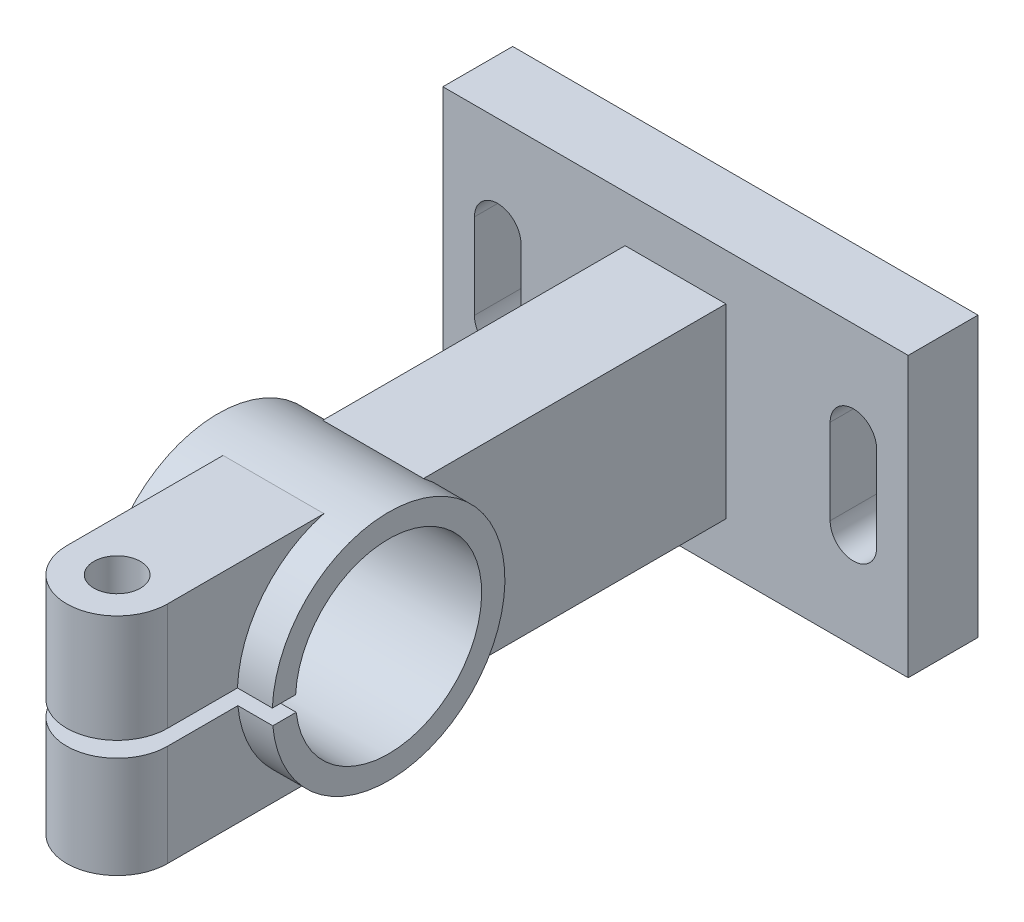
ISO-10303-21;
HEADER;
FILE_DESCRIPTION(('STEP AP214'),'2;1');
FILE_NAME('part.step','',(''),(''),'','','');
FILE_SCHEMA(('AUTOMOTIVE_DESIGN { 1 0 10303 214 1 1 1 1 }'));
ENDSEC;
DATA;
#1=APPLICATION_CONTEXT('core data for automotive mechanical design processes');
#2=APPLICATION_PROTOCOL_DEFINITION('international standard','automotive_design',2000,#1);
#3=PRODUCT_CONTEXT('',#1,'mechanical');
#4=PRODUCT('Part','Part','',(#3));
#5=PRODUCT_RELATED_PRODUCT_CATEGORY('part','',(#4));
#6=PRODUCT_DEFINITION_FORMATION('','',#4);
#7=PRODUCT_DEFINITION_CONTEXT('part definition',#1,'design');
#8=PRODUCT_DEFINITION('design','',#6,#7);
#9=PRODUCT_DEFINITION_SHAPE('','',#8);
#10=(LENGTH_UNIT() NAMED_UNIT(*) SI_UNIT(.MILLI.,.METRE.));
#11=(NAMED_UNIT(*) PLANE_ANGLE_UNIT() SI_UNIT($,.RADIAN.));
#12=(NAMED_UNIT(*) SI_UNIT($,.STERADIAN.) SOLID_ANGLE_UNIT());
#13=UNCERTAINTY_MEASURE_WITH_UNIT(LENGTH_MEASURE(1.E-05),#10,'distance_accuracy_value','');
#14=(GEOMETRIC_REPRESENTATION_CONTEXT(3) GLOBAL_UNCERTAINTY_ASSIGNED_CONTEXT((#13)) GLOBAL_UNIT_ASSIGNED_CONTEXT((#10,
#11,#12)) REPRESENTATION_CONTEXT('',''));
#15=CARTESIAN_POINT('',(0.,0.,0.));
#16=DIRECTION('',(0.,0.,1.));
#17=DIRECTION('',(1.,0.,0.));
#18=AXIS2_PLACEMENT_3D('',#15,#16,#17);
#19=CARTESIAN_POINT('',(0.,0.,9.));
#20=DIRECTION('',(0.,0.,-1.));
#21=DIRECTION('',(-1.,0.,0.));
#22=AXIS2_PLACEMENT_3D('',#19,#20,#21);
#23=PLANE('',#22);
#24=DIRECTION('',(0.,-1.,0.));
#25=VECTOR('',#24,1.);
#26=CARTESIAN_POINT('',(8.13242818806854,47.,9.));
#27=LINE('',#26,#25);
#28=CARTESIAN_POINT('',(8.13242818806854,47.,9.));
#29=VERTEX_POINT('',#28);
#30=CARTESIAN_POINT('',(8.13242818806854,25.,9.));
#31=VERTEX_POINT('',#30);
#32=EDGE_CURVE('E246',#29,#31,#27,.T.);
#33=ORIENTED_EDGE('',*,*,#32,.F.);
#34=CARTESIAN_POINT('',(14.1324281880685,47.,9.));
#35=DIRECTION('',(0.,0.,1.));
#36=DIRECTION('',(1.,0.,0.));
#37=AXIS2_PLACEMENT_3D('',#34,#35,#36);
#38=CIRCLE('',#37,6.);
#39=CARTESIAN_POINT('',(20.1324281880686,47.,9.));
#40=VERTEX_POINT('',#39);
#41=EDGE_CURVE('E58',#40,#29,#38,.T.);
#42=ORIENTED_EDGE('',*,*,#41,.F.);
#43=DIRECTION('',(0.,-1.,0.));
#44=VECTOR('',#43,1.);
#45=CARTESIAN_POINT('',(20.1324281880686,47.,9.));
#46=LINE('',#45,#44);
#47=CARTESIAN_POINT('',(20.1324281880686,25.,9.));
#48=VERTEX_POINT('',#47);
#49=EDGE_CURVE('E255',#40,#48,#46,.T.);
#50=ORIENTED_EDGE('',*,*,#49,.T.);
#51=CARTESIAN_POINT('',(14.1324281880685,25.,9.));
#52=DIRECTION('',(0.,0.,1.));
#53=DIRECTION('',(1.,0.,0.));
#54=AXIS2_PLACEMENT_3D('',#51,#52,#53);
#55=CIRCLE('',#54,6.);
#56=EDGE_CURVE('E236',#31,#48,#55,.T.);
#57=ORIENTED_EDGE('',*,*,#56,.F.);
#58=EDGE_LOOP('',(#33,#42,#50,#57));
#59=FACE_BOUND('',#58,.T.);
#60=DIRECTION('',(0.,-1.,0.));
#61=VECTOR('',#60,1.);
#62=CARTESIAN_POINT('',(47.,60.,9.));
#63=LINE('',#62,#61);
#64=CARTESIAN_POINT('',(47.,60.,9.));
#65=VERTEX_POINT('',#64);
#66=CARTESIAN_POINT('',(47.,12.,9.));
#67=VERTEX_POINT('',#66);
#68=EDGE_CURVE('E381',#65,#67,#63,.T.);
#69=ORIENTED_EDGE('',*,*,#68,.F.);
#70=DIRECTION('',(1.,0.,0.));
#71=VECTOR('',#70,1.);
#72=CARTESIAN_POINT('',(47.,60.,9.));
#73=LINE('',#72,#71);
#74=CARTESIAN_POINT('',(73.,60.,9.));
#75=VERTEX_POINT('',#74);
#76=EDGE_CURVE('E373',#65,#75,#73,.T.);
#77=ORIENTED_EDGE('',*,*,#76,.T.);
#78=DIRECTION('',(0.,-1.,0.));
#79=VECTOR('',#78,1.);
#80=CARTESIAN_POINT('',(73.,60.,9.));
#81=LINE('',#80,#79);
#82=CARTESIAN_POINT('',(73.,12.,9.));
#83=VERTEX_POINT('',#82);
#84=EDGE_CURVE('E374',#75,#83,#81,.T.);
#85=ORIENTED_EDGE('',*,*,#84,.T.);
#86=DIRECTION('',(1.,0.,0.));
#87=VECTOR('',#86,1.);
#88=CARTESIAN_POINT('',(47.,12.,9.));
#89=LINE('',#88,#87);
#90=EDGE_CURVE('E378',#67,#83,#89,.T.);
#91=ORIENTED_EDGE('',*,*,#90,.F.);
#92=EDGE_LOOP('',(#69,#77,#85,#91));
#93=FACE_BOUND('',#92,.T.);
#94=DIRECTION('',(0.,1.,0.));
#95=VECTOR('',#94,1.);
#96=CARTESIAN_POINT('',(0.,0.,9.));
#97=LINE('',#96,#95);
#98=CARTESIAN_POINT('',(0.,0.,9.));
#99=VERTEX_POINT('',#98);
#100=CARTESIAN_POINT('',(0.,72.,9.));
#101=VERTEX_POINT('',#100);
#102=EDGE_CURVE('E403',#99,#101,#97,.T.);
#103=ORIENTED_EDGE('',*,*,#102,.F.);
#104=DIRECTION('',(1.,0.,0.));
#105=VECTOR('',#104,1.);
#106=CARTESIAN_POINT('',(0.,0.,9.));
#107=LINE('',#106,#105);
#108=CARTESIAN_POINT('',(120.,0.,9.));
#109=VERTEX_POINT('',#108);
#110=EDGE_CURVE('E414',#99,#109,#107,.T.);
#111=ORIENTED_EDGE('',*,*,#110,.T.);
#112=DIRECTION('',(0.,1.,0.));
#113=VECTOR('',#112,1.);
#114=CARTESIAN_POINT('',(120.,0.,9.));
#115=LINE('',#114,#113);
#116=CARTESIAN_POINT('',(120.,72.,9.));
#117=VERTEX_POINT('',#116);
#118=EDGE_CURVE('E415',#109,#117,#115,.T.);
#119=ORIENTED_EDGE('',*,*,#118,.T.);
#120=DIRECTION('',(1.,0.,0.));
#121=VECTOR('',#120,1.);
#122=CARTESIAN_POINT('',(0.,72.,9.));
#123=LINE('',#122,#121);
#124=EDGE_CURVE('E409',#101,#117,#123,.T.);
#125=ORIENTED_EDGE('',*,*,#124,.F.);
#126=EDGE_LOOP('',(#103,#111,#119,#125));
#127=FACE_BOUND('',#126,.T.);
#128=CARTESIAN_POINT('',(105.867571811931,47.,9.));
#129=DIRECTION('',(0.,0.,-1.));
#130=DIRECTION('',(-1.,0.,0.));
#131=AXIS2_PLACEMENT_3D('',#128,#129,#130);
#132=CIRCLE('',#131,6.00000000000001);
#133=CARTESIAN_POINT('',(99.8675718119314,47.,9.));
#134=VERTEX_POINT('',#133);
#135=CARTESIAN_POINT('',(111.867571811931,47.,9.));
#136=VERTEX_POINT('',#135);
#137=EDGE_CURVE('E68',#134,#136,#132,.T.);
#138=ORIENTED_EDGE('',*,*,#137,.T.);
#139=DIRECTION('',(0.,-1.,0.));
#140=VECTOR('',#139,1.);
#141=CARTESIAN_POINT('',(111.867571811931,47.,9.));
#142=LINE('',#141,#140);
#143=CARTESIAN_POINT('',(111.867571811931,25.,9.));
#144=VERTEX_POINT('',#143);
#145=EDGE_CURVE('E277',#136,#144,#142,.T.);
#146=ORIENTED_EDGE('',*,*,#145,.T.);
#147=CARTESIAN_POINT('',(105.867571811931,25.,9.));
#148=DIRECTION('',(0.,0.,-1.));
#149=DIRECTION('',(-1.,0.,0.));
#150=AXIS2_PLACEMENT_3D('',#147,#148,#149);
#151=CIRCLE('',#150,6.00000000000001);
#152=CARTESIAN_POINT('',(99.8675718119314,25.,9.));
#153=VERTEX_POINT('',#152);
#154=EDGE_CURVE('E271',#144,#153,#151,.T.);
#155=ORIENTED_EDGE('',*,*,#154,.T.);
#156=DIRECTION('',(0.,-1.,0.));
#157=VECTOR('',#156,1.);
#158=CARTESIAN_POINT('',(99.8675718119314,47.,9.));
#159=LINE('',#158,#157);
#160=EDGE_CURVE('E268',#134,#153,#159,.T.);
#161=ORIENTED_EDGE('',*,*,#160,.F.);
#162=EDGE_LOOP('',(#138,#146,#155,#161));
#163=FACE_BOUND('',#162,.T.);
#164=ADVANCED_FACE('F44',(#59,#93,#127,#163),#23,.F.);
#165=CARTESIAN_POINT('',(0.,0.,-9.));
#166=DIRECTION('',(0.,0.,-1.));
#167=DIRECTION('',(-1.,0.,0.));
#168=AXIS2_PLACEMENT_3D('',#165,#166,#167);
#169=PLANE('',#168);
#170=CARTESIAN_POINT('',(14.1324281880685,47.,-9.));
#171=DIRECTION('',(0.,0.,-1.));
#172=DIRECTION('',(-1.,0.,0.));
#173=AXIS2_PLACEMENT_3D('',#170,#171,#172);
#174=CIRCLE('',#173,6.);
#175=CARTESIAN_POINT('',(8.13242818806854,47.,-9.));
#176=VERTEX_POINT('',#175);
#177=CARTESIAN_POINT('',(20.1324281880686,47.,-9.));
#178=VERTEX_POINT('',#177);
#179=EDGE_CURVE('E12',#176,#178,#174,.T.);
#180=ORIENTED_EDGE('',*,*,#179,.F.);
#181=DIRECTION('',(0.,1.,0.));
#182=VECTOR('',#181,1.);
#183=CARTESIAN_POINT('',(8.13242818806854,0.,-9.));
#184=LINE('',#183,#182);
#185=CARTESIAN_POINT('',(8.13242818806854,25.,-9.));
#186=VERTEX_POINT('',#185);
#187=EDGE_CURVE('E452',#186,#176,#184,.T.);
#188=ORIENTED_EDGE('',*,*,#187,.F.);
#189=CARTESIAN_POINT('',(14.1324281880685,25.,-9.));
#190=DIRECTION('',(0.,0.,-1.));
#191=DIRECTION('',(-1.,0.,0.));
#192=AXIS2_PLACEMENT_3D('',#189,#190,#191);
#193=CIRCLE('',#192,6.);
#194=CARTESIAN_POINT('',(20.1324281880686,25.,-9.));
#195=VERTEX_POINT('',#194);
#196=EDGE_CURVE('E237',#195,#186,#193,.T.);
#197=ORIENTED_EDGE('',*,*,#196,.F.);
#198=DIRECTION('',(0.,1.,0.));
#199=VECTOR('',#198,1.);
#200=CARTESIAN_POINT('',(20.1324281880686,0.,-9.));
#201=LINE('',#200,#199);
#202=EDGE_CURVE('E52',#195,#178,#201,.T.);
#203=ORIENTED_EDGE('',*,*,#202,.T.);
#204=EDGE_LOOP('',(#180,#188,#197,#203));
#205=FACE_BOUND('',#204,.T.);
#206=DIRECTION('',(0.,1.,0.));
#207=VECTOR('',#206,1.);
#208=CARTESIAN_POINT('',(0.,0.,-9.));
#209=LINE('',#208,#207);
#210=CARTESIAN_POINT('',(0.,0.,-9.));
#211=VERTEX_POINT('',#210);
#212=CARTESIAN_POINT('',(0.,72.,-9.));
#213=VERTEX_POINT('',#212);
#214=EDGE_CURVE('E398',#211,#213,#209,.T.);
#215=ORIENTED_EDGE('',*,*,#214,.T.);
#216=DIRECTION('',(1.,0.,0.));
#217=VECTOR('',#216,1.);
#218=CARTESIAN_POINT('',(0.,72.,-9.));
#219=LINE('',#218,#217);
#220=CARTESIAN_POINT('',(120.,72.,-9.));
#221=VERTEX_POINT('',#220);
#222=EDGE_CURVE('E416',#213,#221,#219,.T.);
#223=ORIENTED_EDGE('',*,*,#222,.T.);
#224=DIRECTION('',(0.,1.,0.));
#225=VECTOR('',#224,1.);
#226=CARTESIAN_POINT('',(120.,0.,-9.));
#227=LINE('',#226,#225);
#228=CARTESIAN_POINT('',(120.,0.,-9.));
#229=VERTEX_POINT('',#228);
#230=EDGE_CURVE('E422',#229,#221,#227,.T.);
#231=ORIENTED_EDGE('',*,*,#230,.F.);
#232=DIRECTION('',(1.,0.,0.));
#233=VECTOR('',#232,1.);
#234=CARTESIAN_POINT('',(0.,0.,-9.));
#235=LINE('',#234,#233);
#236=EDGE_CURVE('E406',#211,#229,#235,.T.);
#237=ORIENTED_EDGE('',*,*,#236,.F.);
#238=EDGE_LOOP('',(#215,#223,#231,#237));
#239=FACE_BOUND('',#238,.T.);
#240=DIRECTION('',(0.,1.,0.));
#241=VECTOR('',#240,1.);
#242=CARTESIAN_POINT('',(111.867571811931,0.,-9.));
#243=LINE('',#242,#241);
#244=CARTESIAN_POINT('',(111.867571811931,25.,-9.));
#245=VERTEX_POINT('',#244);
#246=CARTESIAN_POINT('',(111.867571811931,47.,-9.));
#247=VERTEX_POINT('',#246);
#248=EDGE_CURVE('E444',#245,#247,#243,.T.);
#249=ORIENTED_EDGE('',*,*,#248,.T.);
#250=CARTESIAN_POINT('',(105.867571811931,47.,-9.));
#251=DIRECTION('',(0.,0.,-1.));
#252=DIRECTION('',(-1.,0.,0.));
#253=AXIS2_PLACEMENT_3D('',#250,#251,#252);
#254=CIRCLE('',#253,6.00000000000001);
#255=CARTESIAN_POINT('',(99.8675718119314,47.,-9.));
#256=VERTEX_POINT('',#255);
#257=EDGE_CURVE('E449',#247,#256,#254,.F.);
#258=ORIENTED_EDGE('',*,*,#257,.T.);
#259=DIRECTION('',(0.,1.,0.));
#260=VECTOR('',#259,1.);
#261=CARTESIAN_POINT('',(99.8675718119314,0.,-9.));
#262=LINE('',#261,#260);
#263=CARTESIAN_POINT('',(99.8675718119314,25.,-9.));
#264=VERTEX_POINT('',#263);
#265=EDGE_CURVE('E426',#264,#256,#262,.T.);
#266=ORIENTED_EDGE('',*,*,#265,.F.);
#267=CARTESIAN_POINT('',(105.867571811931,25.,-9.));
#268=DIRECTION('',(0.,0.,-1.));
#269=DIRECTION('',(-1.,0.,0.));
#270=AXIS2_PLACEMENT_3D('',#267,#268,#269);
#271=CIRCLE('',#270,6.00000000000001);
#272=EDGE_CURVE('E445',#264,#245,#271,.F.);
#273=ORIENTED_EDGE('',*,*,#272,.T.);
#274=EDGE_LOOP('',(#249,#258,#266,#273));
#275=FACE_BOUND('',#274,.T.);
#276=ADVANCED_FACE('F457',(#205,#239,#275),#169,.T.);
#277=CARTESIAN_POINT('',(73.,36.,105.));
#278=DIRECTION('',(1.,0.,0.));
#279=DIRECTION('',(0.,0.,-1.));
#280=AXIS2_PLACEMENT_3D('',#277,#278,#279);
#281=PLANE('',#280);
#282=DIRECTION('',(0.,0.,-1.));
#283=VECTOR('',#282,1.);
#284=CARTESIAN_POINT('',(73.,33.2118861874641,105.));
#285=LINE('',#284,#283);
#286=CARTESIAN_POINT('',(73.,33.2118861874641,153.));
#287=VERTEX_POINT('',#286);
#288=CARTESIAN_POINT('',(73.,33.2118861874641,134.870159379694));
#289=VERTEX_POINT('',#288);
#290=EDGE_CURVE('E307',#287,#289,#285,.T.);
#291=ORIENTED_EDGE('',*,*,#290,.F.);
#292=DIRECTION('',(0.,1.,0.));
#293=VECTOR('',#292,1.);
#294=CARTESIAN_POINT('',(73.,7.,153.));
#295=LINE('',#294,#293);
#296=CARTESIAN_POINT('',(73.,7.,153.));
#297=VERTEX_POINT('',#296);
#298=EDGE_CURVE('E338',#297,#287,#295,.T.);
#299=ORIENTED_EDGE('',*,*,#298,.F.);
#300=DIRECTION('',(0.,0.,-1.));
#301=VECTOR('',#300,1.);
#302=CARTESIAN_POINT('',(73.,7.,153.));
#303=LINE('',#302,#301);
#304=CARTESIAN_POINT('',(73.,6.99999999999999,112.681145747869));
#305=VERTEX_POINT('',#304);
#306=EDGE_CURVE('E328',#297,#305,#303,.T.);
#307=ORIENTED_EDGE('',*,*,#306,.T.);
#308=CARTESIAN_POINT('',(73.,36.,105.));
#309=DIRECTION('',(1.,0.,0.));
#310=DIRECTION('',(0.,0.,-1.));
#311=AXIS2_PLACEMENT_3D('',#308,#309,#310);
#312=CIRCLE('',#311,30.);
#313=EDGE_CURVE('E332',#289,#305,#312,.T.);
#314=ORIENTED_EDGE('',*,*,#313,.F.);
#315=EDGE_LOOP('',(#291,#299,#307,#314));
#316=FACE_BOUND('',#315,.T.);
#317=ADVANCED_FACE('F482',(#316),#281,.T.);
#318=CARTESIAN_POINT('',(47.,36.,105.));
#319=DIRECTION('',(1.,0.,0.));
#320=DIRECTION('',(0.,0.,-1.));
#321=AXIS2_PLACEMENT_3D('',#318,#319,#320);
#322=PLANE('',#321);
#323=DIRECTION('',(0.,1.,0.));
#324=VECTOR('',#323,1.);
#325=CARTESIAN_POINT('',(47.,7.,153.));
#326=LINE('',#325,#324);
#327=CARTESIAN_POINT('',(47.,7.,153.));
#328=VERTEX_POINT('',#327);
#329=CARTESIAN_POINT('',(47.,33.2118861874641,153.));
#330=VERTEX_POINT('',#329);
#331=EDGE_CURVE('E335',#328,#330,#326,.T.);
#332=ORIENTED_EDGE('',*,*,#331,.T.);
#333=DIRECTION('',(0.,0.,-1.));
#334=VECTOR('',#333,1.);
#335=CARTESIAN_POINT('',(47.,33.2118861874641,105.));
#336=LINE('',#335,#334);
#337=CARTESIAN_POINT('',(47.,33.2118861874641,134.870159379694));
#338=VERTEX_POINT('',#337);
#339=EDGE_CURVE('E306',#330,#338,#336,.T.);
#340=ORIENTED_EDGE('',*,*,#339,.T.);
#341=CARTESIAN_POINT('',(47.,36.,105.));
#342=DIRECTION('',(1.,0.,0.));
#343=DIRECTION('',(0.,0.,-1.));
#344=AXIS2_PLACEMENT_3D('',#341,#342,#343);
#345=CIRCLE('',#344,30.);
#346=CARTESIAN_POINT('',(47.,6.99999999999999,112.681145747869));
#347=VERTEX_POINT('',#346);
#348=EDGE_CURVE('E347',#338,#347,#345,.T.);
#349=ORIENTED_EDGE('',*,*,#348,.T.);
#350=DIRECTION('',(0.,0.,-1.));
#351=VECTOR('',#350,1.);
#352=CARTESIAN_POINT('',(47.,7.,153.));
#353=LINE('',#352,#351);
#354=EDGE_CURVE('E321',#328,#347,#353,.T.);
#355=ORIENTED_EDGE('',*,*,#354,.F.);
#356=EDGE_LOOP('',(#332,#340,#349,#355));
#357=FACE_BOUND('',#356,.T.);
#358=ADVANCED_FACE('F557',(#357),#322,.F.);
#359=CARTESIAN_POINT('',(60.,65.,153.));
#360=DIRECTION('',(0.,-1.,0.));
#361=DIRECTION('',(0.,0.,-1.));
#362=AXIS2_PLACEMENT_3D('',#359,#360,#361);
#363=CYLINDRICAL_SURFACE('',#362,13.);
#364=CARTESIAN_POINT('',(47.,37.2118861874641,153.));
#365=VERTEX_POINT('',#364);
#366=CARTESIAN_POINT('',(47.,65.,153.));
#367=VERTEX_POINT('',#366);
#368=EDGE_CURVE('E355',#365,#367,#326,.T.);
#369=ORIENTED_EDGE('',*,*,#368,.F.);
#370=CARTESIAN_POINT('',(60.,37.2118861874641,153.));
#371=DIRECTION('',(0.,1.,0.));
#372=DIRECTION('',(0.,0.,1.));
#373=AXIS2_PLACEMENT_3D('',#370,#371,#372);
#374=CIRCLE('',#373,13.);
#375=CARTESIAN_POINT('',(73.,37.2118861874641,153.));
#376=VERTEX_POINT('',#375);
#377=EDGE_CURVE('E288',#376,#365,#374,.F.);
#378=ORIENTED_EDGE('',*,*,#377,.F.);
#379=CARTESIAN_POINT('',(73.,65.,153.));
#380=VERTEX_POINT('',#379);
#381=EDGE_CURVE('E339',#376,#380,#295,.T.);
#382=ORIENTED_EDGE('',*,*,#381,.T.);
#383=CARTESIAN_POINT('',(60.,65.,153.));
#384=DIRECTION('',(0.,-1.,0.));
#385=DIRECTION('',(0.,0.,-1.));
#386=AXIS2_PLACEMENT_3D('',#383,#384,#385);
#387=CIRCLE('',#386,13.);
#388=EDGE_CURVE('E322',#380,#367,#387,.T.);
#389=ORIENTED_EDGE('',*,*,#388,.T.);
#390=EDGE_LOOP('',(#369,#378,#382,#389));
#391=FACE_BOUND('',#390,.T.);
#392=ADVANCED_FACE('F553',(#391),#363,.T.);
#393=CARTESIAN_POINT('',(60.,85.,153.));
#394=DIRECTION('',(0.,-1.,0.));
#395=DIRECTION('',(0.,0.,-1.));
#396=AXIS2_PLACEMENT_3D('',#393,#394,#395);
#397=CYLINDRICAL_SURFACE('',#396,6.);
#398=CARTESIAN_POINT('',(60.,33.2118861874641,153.));
#399=DIRECTION('',(0.,-1.,0.));
#400=DIRECTION('',(0.,0.,-1.));
#401=AXIS2_PLACEMENT_3D('',#398,#399,#400);
#402=CIRCLE('',#401,6.);
#403=CARTESIAN_POINT('',(60.,33.2118861874641,147.));
#404=VERTEX_POINT('',#403);
#405=EDGE_CURVE('E303',#404,#404,#402,.F.);
#406=ORIENTED_EDGE('',*,*,#405,.T.);
#407=EDGE_LOOP('',(#406));
#408=FACE_BOUND('',#407,.T.);
#409=CARTESIAN_POINT('',(60.,7.,153.));
#410=DIRECTION('',(0.,-1.,0.));
#411=DIRECTION('',(0.,0.,-1.));
#412=AXIS2_PLACEMENT_3D('',#409,#410,#411);
#413=CIRCLE('',#412,6.);
#414=CARTESIAN_POINT('',(60.,7.,147.));
#415=VERTEX_POINT('',#414);
#416=EDGE_CURVE('E320',#415,#415,#413,.T.);
#417=ORIENTED_EDGE('',*,*,#416,.T.);
#418=EDGE_LOOP('',(#417));
#419=FACE_BOUND('',#418,.T.);
#420=ADVANCED_FACE('F547',(#408,#419),#397,.F.);
#421=CARTESIAN_POINT('',(0.,0.,9.));
#422=DIRECTION('',(-1.,0.,0.));
#423=DIRECTION('',(0.,0.,1.));
#424=AXIS2_PLACEMENT_3D('',#421,#422,#423);
#425=PLANE('',#424);
#426=ORIENTED_EDGE('',*,*,#214,.F.);
#427=DIRECTION('',(0.,0.,-1.));
#428=VECTOR('',#427,1.);
#429=CARTESIAN_POINT('',(0.,0.,9.));
#430=LINE('',#429,#428);
#431=EDGE_CURVE('E428',#99,#211,#430,.T.);
#432=ORIENTED_EDGE('',*,*,#431,.F.);
#433=ORIENTED_EDGE('',*,*,#102,.T.);
#434=DIRECTION('',(0.,0.,-1.));
#435=VECTOR('',#434,1.);
#436=CARTESIAN_POINT('',(0.,72.,9.));
#437=LINE('',#436,#435);
#438=EDGE_CURVE('E417',#101,#213,#437,.T.);
#439=ORIENTED_EDGE('',*,*,#438,.T.);
#440=EDGE_LOOP('',(#426,#432,#433,#439));
#441=FACE_BOUND('',#440,.T.);
#442=ADVANCED_FACE('F50',(#441),#425,.T.);
#443=CARTESIAN_POINT('',(0.,0.,9.));
#444=DIRECTION('',(0.,1.,0.));
#445=DIRECTION('',(0.,0.,1.));
#446=AXIS2_PLACEMENT_3D('',#443,#444,#445);
#447=PLANE('',#446);
#448=ORIENTED_EDGE('',*,*,#236,.T.);
#449=DIRECTION('',(0.,0.,-1.));
#450=VECTOR('',#449,1.);
#451=CARTESIAN_POINT('',(120.,0.,9.));
#452=LINE('',#451,#450);
#453=EDGE_CURVE('E429',#109,#229,#452,.T.);
#454=ORIENTED_EDGE('',*,*,#453,.F.);
#455=ORIENTED_EDGE('',*,*,#110,.F.);
#456=ORIENTED_EDGE('',*,*,#431,.T.);
#457=EDGE_LOOP('',(#448,#454,#455,#456));
#458=FACE_BOUND('',#457,.T.);
#459=ADVANCED_FACE('F487',(#458),#447,.F.);
#460=CARTESIAN_POINT('',(120.,0.,9.));
#461=DIRECTION('',(-1.,0.,0.));
#462=DIRECTION('',(0.,0.,1.));
#463=AXIS2_PLACEMENT_3D('',#460,#461,#462);
#464=PLANE('',#463);
#465=ORIENTED_EDGE('',*,*,#230,.T.);
#466=DIRECTION('',(0.,0.,-1.));
#467=VECTOR('',#466,1.);
#468=CARTESIAN_POINT('',(120.,72.,9.));
#469=LINE('',#468,#467);
#470=EDGE_CURVE('E435',#117,#221,#469,.T.);
#471=ORIENTED_EDGE('',*,*,#470,.F.);
#472=ORIENTED_EDGE('',*,*,#118,.F.);
#473=ORIENTED_EDGE('',*,*,#453,.T.);
#474=EDGE_LOOP('',(#465,#471,#472,#473));
#475=FACE_BOUND('',#474,.T.);
#476=ADVANCED_FACE('F489',(#475),#464,.F.);
#477=CARTESIAN_POINT('',(0.,72.,9.));
#478=DIRECTION('',(0.,1.,0.));
#479=DIRECTION('',(0.,0.,1.));
#480=AXIS2_PLACEMENT_3D('',#477,#478,#479);
#481=PLANE('',#480);
#482=ORIENTED_EDGE('',*,*,#222,.F.);
#483=ORIENTED_EDGE('',*,*,#438,.F.);
#484=ORIENTED_EDGE('',*,*,#124,.T.);
#485=ORIENTED_EDGE('',*,*,#470,.T.);
#486=EDGE_LOOP('',(#482,#483,#484,#485));
#487=FACE_BOUND('',#486,.T.);
#488=ADVANCED_FACE('F491',(#487),#481,.T.);
#489=CARTESIAN_POINT('',(47.,12.,135.001));
#490=DIRECTION('',(0.,1.,0.));
#491=DIRECTION('',(0.,0.,1.));
#492=AXIS2_PLACEMENT_3D('',#489,#490,#491);
#493=PLANE('',#492);
#494=DIRECTION('',(0.,0.,-1.));
#495=VECTOR('',#494,1.);
#496=CARTESIAN_POINT('',(73.,12.,135.001));
#497=LINE('',#496,#495);
#498=CARTESIAN_POINT('',(73.,12.,87.));
#499=VERTEX_POINT('',#498);
#500=EDGE_CURVE('E376',#499,#83,#497,.T.);
#501=ORIENTED_EDGE('',*,*,#500,.F.);
#502=DIRECTION('',(-1.,0.,0.));
#503=VECTOR('',#502,1.);
#504=CARTESIAN_POINT('',(82.,12.,87.));
#505=LINE('',#504,#503);
#506=CARTESIAN_POINT('',(47.,12.,87.));
#507=VERTEX_POINT('',#506);
#508=EDGE_CURVE('E369',#499,#507,#505,.T.);
#509=ORIENTED_EDGE('',*,*,#508,.T.);
#510=DIRECTION('',(0.,0.,-1.));
#511=VECTOR('',#510,1.);
#512=CARTESIAN_POINT('',(47.,12.,135.001));
#513=LINE('',#512,#511);
#514=EDGE_CURVE('E384',#507,#67,#513,.T.);
#515=ORIENTED_EDGE('',*,*,#514,.T.);
#516=ORIENTED_EDGE('',*,*,#90,.T.);
#517=EDGE_LOOP('',(#501,#509,#515,#516));
#518=FACE_BOUND('',#517,.T.);
#519=ADVANCED_FACE('F496',(#518),#493,.F.);
#520=CARTESIAN_POINT('',(47.,60.,135.001));
#521=DIRECTION('',(0.,1.,0.));
#522=DIRECTION('',(-1.,0.,0.));
#523=AXIS2_PLACEMENT_3D('',#520,#521,#522);
#524=PLANE('',#523);
#525=DIRECTION('',(-1.,0.,0.));
#526=VECTOR('',#525,1.);
#527=CARTESIAN_POINT('',(82.,60.,87.));
#528=LINE('',#527,#526);
#529=CARTESIAN_POINT('',(73.,60.,87.));
#530=VERTEX_POINT('',#529);
#531=CARTESIAN_POINT('',(47.,60.,87.));
#532=VERTEX_POINT('',#531);
#533=EDGE_CURVE('E400',#530,#532,#528,.T.);
#534=ORIENTED_EDGE('',*,*,#533,.F.);
#535=DIRECTION('',(0.,0.,-1.));
#536=VECTOR('',#535,1.);
#537=CARTESIAN_POINT('',(73.,60.,135.001));
#538=LINE('',#537,#536);
#539=EDGE_CURVE('E385',#530,#75,#538,.T.);
#540=ORIENTED_EDGE('',*,*,#539,.T.);
#541=ORIENTED_EDGE('',*,*,#76,.F.);
#542=DIRECTION('',(0.,0.,-1.));
#543=VECTOR('',#542,1.);
#544=CARTESIAN_POINT('',(47.,60.,135.001));
#545=LINE('',#544,#543);
#546=EDGE_CURVE('E390',#532,#65,#545,.T.);
#547=ORIENTED_EDGE('',*,*,#546,.F.);
#548=EDGE_LOOP('',(#534,#540,#541,#547));
#549=FACE_BOUND('',#548,.T.);
#550=ADVANCED_FACE('F481',(#549),#524,.T.);
#551=CARTESIAN_POINT('',(47.,60.,135.001));
#552=DIRECTION('',(1.,0.,0.));
#553=DIRECTION('',(0.,1.,0.));
#554=AXIS2_PLACEMENT_3D('',#551,#552,#553);
#555=PLANE('',#554);
#556=ORIENTED_EDGE('',*,*,#514,.F.);
#557=CARTESIAN_POINT('',(47.,36.,105.));
#558=DIRECTION('',(1.,0.,0.));
#559=DIRECTION('',(0.,1.,0.));
#560=AXIS2_PLACEMENT_3D('',#557,#558,#559);
#561=CIRCLE('',#560,30.);
#562=EDGE_CURVE('E394',#507,#532,#561,.T.);
#563=ORIENTED_EDGE('',*,*,#562,.T.);
#564=ORIENTED_EDGE('',*,*,#546,.T.);
#565=ORIENTED_EDGE('',*,*,#68,.T.);
#566=EDGE_LOOP('',(#556,#563,#564,#565));
#567=FACE_BOUND('',#566,.T.);
#568=ADVANCED_FACE('F590',(#567),#555,.F.);
#569=CARTESIAN_POINT('',(73.,60.,135.001));
#570=DIRECTION('',(1.,0.,0.));
#571=DIRECTION('',(0.,0.,-1.));
#572=AXIS2_PLACEMENT_3D('',#569,#570,#571);
#573=PLANE('',#572);
#574=CARTESIAN_POINT('',(73.,36.,105.));
#575=DIRECTION('',(1.,0.,0.));
#576=DIRECTION('',(0.,0.,-1.));
#577=AXIS2_PLACEMENT_3D('',#574,#575,#576);
#578=CIRCLE('',#577,30.);
#579=EDGE_CURVE('E377',#499,#530,#578,.T.);
#580=ORIENTED_EDGE('',*,*,#579,.F.);
#581=ORIENTED_EDGE('',*,*,#500,.T.);
#582=ORIENTED_EDGE('',*,*,#84,.F.);
#583=ORIENTED_EDGE('',*,*,#539,.F.);
#584=EDGE_LOOP('',(#580,#581,#582,#583));
#585=FACE_BOUND('',#584,.T.);
#586=ADVANCED_FACE('F584',(#585),#573,.T.);
#587=CARTESIAN_POINT('',(82.,36.,105.));
#588=DIRECTION('',(-1.,0.,0.));
#589=DIRECTION('',(0.,0.,1.));
#590=AXIS2_PLACEMENT_3D('',#587,#588,#589);
#591=CYLINDRICAL_SURFACE('',#590,30.);
#592=DIRECTION('',(-1.,0.,0.));
#593=VECTOR('',#592,1.);
#594=CARTESIAN_POINT('',(82.,33.2118861874641,134.870159379694));
#595=LINE('',#594,#593);
#596=CARTESIAN_POINT('',(38.,33.2118861874641,134.870159379694));
#597=VERTEX_POINT('',#596);
#598=EDGE_CURVE('E312',#597,#338,#595,.F.);
#599=ORIENTED_EDGE('',*,*,#598,.F.);
#600=CARTESIAN_POINT('',(38.,36.,105.));
#601=DIRECTION('',(-1.,0.,0.));
#602=DIRECTION('',(0.,0.,1.));
#603=AXIS2_PLACEMENT_3D('',#600,#601,#602);
#604=CIRCLE('',#603,30.);
#605=CARTESIAN_POINT('',(38.,37.2118861874641,134.975512203608));
#606=VERTEX_POINT('',#605);
#607=EDGE_CURVE('E364',#606,#597,#604,.T.);
#608=ORIENTED_EDGE('',*,*,#607,.F.);
#609=DIRECTION('',(-1.,0.,0.));
#610=VECTOR('',#609,1.);
#611=CARTESIAN_POINT('',(82.,37.2118861874641,134.975512203608));
#612=LINE('',#611,#610);
#613=CARTESIAN_POINT('',(47.,37.2118861874641,134.975512203608));
#614=VERTEX_POINT('',#613);
#615=EDGE_CURVE('E300',#614,#606,#612,.T.);
#616=ORIENTED_EDGE('',*,*,#615,.F.);
#617=CARTESIAN_POINT('',(47.,65.,112.681145747869));
#618=VERTEX_POINT('',#617);
#619=EDGE_CURVE('E350',#618,#614,#345,.T.);
#620=ORIENTED_EDGE('',*,*,#619,.F.);
#621=DIRECTION('',(-1.,0.,0.));
#622=VECTOR('',#621,1.);
#623=CARTESIAN_POINT('',(73.,65.,112.681145747869));
#624=LINE('',#623,#622);
#625=CARTESIAN_POINT('',(73.,65.,112.681145747869));
#626=VERTEX_POINT('',#625);
#627=EDGE_CURVE('E344',#626,#618,#624,.T.);
#628=ORIENTED_EDGE('',*,*,#627,.F.);
#629=CARTESIAN_POINT('',(73.,37.2118861874641,134.975512203608));
#630=VERTEX_POINT('',#629);
#631=EDGE_CURVE('E334',#626,#630,#312,.T.);
#632=ORIENTED_EDGE('',*,*,#631,.T.);
#633=CARTESIAN_POINT('',(82.,37.2118861874641,134.975512203608));
#634=VERTEX_POINT('',#633);
#635=EDGE_CURVE('E299',#634,#630,#612,.T.);
#636=ORIENTED_EDGE('',*,*,#635,.F.);
#637=CARTESIAN_POINT('',(82.,36.,105.));
#638=DIRECTION('',(-1.,0.,0.));
#639=DIRECTION('',(0.,0.,1.));
#640=AXIS2_PLACEMENT_3D('',#637,#638,#639);
#641=CIRCLE('',#640,30.);
#642=CARTESIAN_POINT('',(82.,33.2118861874641,134.870159379694));
#643=VERTEX_POINT('',#642);
#644=EDGE_CURVE('E370',#634,#643,#641,.T.);
#645=ORIENTED_EDGE('',*,*,#644,.T.);
#646=EDGE_CURVE('E311',#289,#643,#595,.F.);
#647=ORIENTED_EDGE('',*,*,#646,.F.);
#648=ORIENTED_EDGE('',*,*,#313,.T.);
#649=DIRECTION('',(-1.,0.,0.));
#650=VECTOR('',#649,1.);
#651=CARTESIAN_POINT('',(73.,6.99999999999999,112.681145747869));
#652=LINE('',#651,#650);
#653=EDGE_CURVE('E357',#305,#347,#652,.T.);
#654=ORIENTED_EDGE('',*,*,#653,.T.);
#655=ORIENTED_EDGE('',*,*,#348,.F.);
#656=EDGE_LOOP('',(#599,#608,#616,#620,#628,#632,#636,#645,#647,#648,#654,#655));
#657=FACE_BOUND('',#656,.T.);
#658=ORIENTED_EDGE('',*,*,#562,.F.);
#659=ORIENTED_EDGE('',*,*,#508,.F.);
#660=ORIENTED_EDGE('',*,*,#579,.T.);
#661=ORIENTED_EDGE('',*,*,#533,.T.);
#662=EDGE_LOOP('',(#658,#659,#660,#661));
#663=FACE_BOUND('',#662,.T.);
#664=ADVANCED_FACE('F577',(#657,#663),#591,.T.);
#665=CARTESIAN_POINT('',(82.,36.,105.));
#666=DIRECTION('',(-1.,0.,0.));
#667=DIRECTION('',(0.,0.,1.));
#668=AXIS2_PLACEMENT_3D('',#665,#666,#667);
#669=PLANE('',#668);
#670=CARTESIAN_POINT('',(82.,36.,105.));
#671=DIRECTION('',(-1.,0.,0.));
#672=DIRECTION('',(0.,0.,1.));
#673=AXIS2_PLACEMENT_3D('',#670,#671,#672);
#674=CIRCLE('',#673,24.);
#675=CARTESIAN_POINT('',(82.,37.2118861874641,128.969383218361));
#676=VERTEX_POINT('',#675);
#677=CARTESIAN_POINT('',(82.,33.2118861874641,128.837500317113));
#678=VERTEX_POINT('',#677);
#679=EDGE_CURVE('E363',#676,#678,#674,.T.);
#680=ORIENTED_EDGE('',*,*,#679,.T.);
#681=DIRECTION('',(0.,0.,1.));
#682=VECTOR('',#681,1.);
#683=CARTESIAN_POINT('',(82.,33.2118861874641,88.));
#684=LINE('',#683,#682);
#685=EDGE_CURVE('E278',#678,#643,#684,.T.);
#686=ORIENTED_EDGE('',*,*,#685,.T.);
#687=ORIENTED_EDGE('',*,*,#644,.F.);
#688=DIRECTION('',(0.,0.,1.));
#689=VECTOR('',#688,1.);
#690=CARTESIAN_POINT('',(82.,37.2118861874641,88.));
#691=LINE('',#690,#689);
#692=EDGE_CURVE('E256',#676,#634,#691,.T.);
#693=ORIENTED_EDGE('',*,*,#692,.F.);
#694=EDGE_LOOP('',(#680,#686,#687,#693));
#695=FACE_BOUND('',#694,.T.);
#696=ADVANCED_FACE('F572',(#695),#669,.F.);
#697=CARTESIAN_POINT('',(38.,36.,105.));
#698=DIRECTION('',(-1.,0.,0.));
#699=DIRECTION('',(0.,0.,1.));
#700=AXIS2_PLACEMENT_3D('',#697,#698,#699);
#701=PLANE('',#700);
#702=DIRECTION('',(0.,0.,1.));
#703=VECTOR('',#702,1.);
#704=CARTESIAN_POINT('',(38.,33.2118861874641,88.));
#705=LINE('',#704,#703);
#706=CARTESIAN_POINT('',(38.,33.2118861874641,128.837500317113));
#707=VERTEX_POINT('',#706);
#708=EDGE_CURVE('E284',#707,#597,#705,.T.);
#709=ORIENTED_EDGE('',*,*,#708,.F.);
#710=CARTESIAN_POINT('',(38.,36.,105.));
#711=DIRECTION('',(-1.,0.,0.));
#712=DIRECTION('',(0.,0.,1.));
#713=AXIS2_PLACEMENT_3D('',#710,#711,#712);
#714=CIRCLE('',#713,24.);
#715=CARTESIAN_POINT('',(38.,37.2118861874641,128.969383218361));
#716=VERTEX_POINT('',#715);
#717=EDGE_CURVE('E359',#716,#707,#714,.T.);
#718=ORIENTED_EDGE('',*,*,#717,.F.);
#719=DIRECTION('',(0.,0.,1.));
#720=VECTOR('',#719,1.);
#721=CARTESIAN_POINT('',(38.,37.2118861874641,88.));
#722=LINE('',#721,#720);
#723=EDGE_CURVE('E287',#716,#606,#722,.T.);
#724=ORIENTED_EDGE('',*,*,#723,.T.);
#725=ORIENTED_EDGE('',*,*,#607,.T.);
#726=EDGE_LOOP('',(#709,#718,#724,#725));
#727=FACE_BOUND('',#726,.T.);
#728=ADVANCED_FACE('F571',(#727),#701,.T.);
#729=CARTESIAN_POINT('',(82.,36.,105.));
#730=DIRECTION('',(-1.,0.,0.));
#731=DIRECTION('',(0.,0.,1.));
#732=AXIS2_PLACEMENT_3D('',#729,#730,#731);
#733=CYLINDRICAL_SURFACE('',#732,24.);
#734=ORIENTED_EDGE('',*,*,#717,.T.);
#735=DIRECTION('',(-1.,0.,0.));
#736=VECTOR('',#735,1.);
#737=CARTESIAN_POINT('',(82.,33.2118861874641,128.837500317113));
#738=LINE('',#737,#736);
#739=EDGE_CURVE('E313',#707,#678,#738,.F.);
#740=ORIENTED_EDGE('',*,*,#739,.T.);
#741=ORIENTED_EDGE('',*,*,#679,.F.);
#742=DIRECTION('',(-1.,0.,0.));
#743=VECTOR('',#742,1.);
#744=CARTESIAN_POINT('',(82.,37.2118861874641,128.969383218361));
#745=LINE('',#744,#743);
#746=EDGE_CURVE('E297',#676,#716,#745,.T.);
#747=ORIENTED_EDGE('',*,*,#746,.T.);
#748=EDGE_LOOP('',(#734,#740,#741,#747));
#749=FACE_BOUND('',#748,.T.);
#750=ADVANCED_FACE('F570',(#749),#733,.F.);
#751=CARTESIAN_POINT('',(73.,7.,153.));
#752=DIRECTION('',(0.,1.,0.));
#753=DIRECTION('',(0.,0.,1.));
#754=AXIS2_PLACEMENT_3D('',#751,#752,#753);
#755=PLANE('',#754);
#756=ORIENTED_EDGE('',*,*,#416,.F.);
#757=EDGE_LOOP('',(#756));
#758=FACE_BOUND('',#757,.T.);
#759=ORIENTED_EDGE('',*,*,#354,.T.);
#760=ORIENTED_EDGE('',*,*,#653,.F.);
#761=ORIENTED_EDGE('',*,*,#306,.F.);
#762=CARTESIAN_POINT('',(60.,7.,153.));
#763=DIRECTION('',(0.,-1.,0.));
#764=DIRECTION('',(0.,0.,-1.));
#765=AXIS2_PLACEMENT_3D('',#762,#763,#764);
#766=CIRCLE('',#765,13.);
#767=EDGE_CURVE('E323',#297,#328,#766,.T.);
#768=ORIENTED_EDGE('',*,*,#767,.T.);
#769=EDGE_LOOP('',(#759,#760,#761,#768));
#770=FACE_BOUND('',#769,.T.);
#771=ADVANCED_FACE('F563',(#758,#770),#755,.F.);
#772=CARTESIAN_POINT('',(73.,65.,153.));
#773=DIRECTION('',(0.,1.,0.));
#774=DIRECTION('',(0.,0.,1.));
#775=AXIS2_PLACEMENT_3D('',#772,#773,#774);
#776=PLANE('',#775);
#777=CARTESIAN_POINT('',(60.,65.,153.));
#778=DIRECTION('',(0.,1.,0.));
#779=DIRECTION('',(0.,0.,1.));
#780=AXIS2_PLACEMENT_3D('',#777,#778,#779);
#781=CIRCLE('',#780,6.);
#782=CARTESIAN_POINT('',(60.,65.,159.));
#783=VERTEX_POINT('',#782);
#784=EDGE_CURVE('E318',#783,#783,#781,.T.);
#785=ORIENTED_EDGE('',*,*,#784,.F.);
#786=EDGE_LOOP('',(#785));
#787=FACE_BOUND('',#786,.T.);
#788=DIRECTION('',(0.,0.,-1.));
#789=VECTOR('',#788,1.);
#790=CARTESIAN_POINT('',(47.,65.,153.));
#791=LINE('',#790,#789);
#792=EDGE_CURVE('E346',#367,#618,#791,.T.);
#793=ORIENTED_EDGE('',*,*,#792,.F.);
#794=ORIENTED_EDGE('',*,*,#388,.F.);
#795=DIRECTION('',(0.,0.,-1.));
#796=VECTOR('',#795,1.);
#797=CARTESIAN_POINT('',(73.,65.,153.));
#798=LINE('',#797,#796);
#799=EDGE_CURVE('E337',#380,#626,#798,.T.);
#800=ORIENTED_EDGE('',*,*,#799,.T.);
#801=ORIENTED_EDGE('',*,*,#627,.T.);
#802=EDGE_LOOP('',(#793,#794,#800,#801));
#803=FACE_BOUND('',#802,.T.);
#804=ADVANCED_FACE('F554',(#787,#803),#776,.T.);
#805=DIRECTION('',(0.,0.,1.));
#806=VECTOR('',#805,1.);
#807=CARTESIAN_POINT('',(73.,37.2118861874641,105.));
#808=LINE('',#807,#806);
#809=EDGE_CURVE('E294',#630,#376,#808,.T.);
#810=ORIENTED_EDGE('',*,*,#809,.F.);
#811=ORIENTED_EDGE('',*,*,#631,.F.);
#812=ORIENTED_EDGE('',*,*,#799,.F.);
#813=ORIENTED_EDGE('',*,*,#381,.F.);
#814=EDGE_LOOP('',(#810,#811,#812,#813));
#815=FACE_BOUND('',#814,.T.);
#816=ADVANCED_FACE('F552',(#815),#281,.T.);
#817=ORIENTED_EDGE('',*,*,#619,.T.);
#818=DIRECTION('',(0.,0.,1.));
#819=VECTOR('',#818,1.);
#820=CARTESIAN_POINT('',(47.,37.2118861874641,105.));
#821=LINE('',#820,#819);
#822=EDGE_CURVE('E292',#614,#365,#821,.T.);
#823=ORIENTED_EDGE('',*,*,#822,.T.);
#824=ORIENTED_EDGE('',*,*,#368,.T.);
#825=ORIENTED_EDGE('',*,*,#792,.T.);
#826=EDGE_LOOP('',(#817,#823,#824,#825));
#827=FACE_BOUND('',#826,.T.);
#828=ADVANCED_FACE('F546',(#827),#322,.F.);
#829=ORIENTED_EDGE('',*,*,#298,.T.);
#830=CARTESIAN_POINT('',(60.,33.2118861874641,153.));
#831=DIRECTION('',(0.,-1.,0.));
#832=DIRECTION('',(0.,0.,-1.));
#833=AXIS2_PLACEMENT_3D('',#830,#831,#832);
#834=CIRCLE('',#833,13.);
#835=EDGE_CURVE('E302',#330,#287,#834,.F.);
#836=ORIENTED_EDGE('',*,*,#835,.F.);
#837=ORIENTED_EDGE('',*,*,#331,.F.);
#838=ORIENTED_EDGE('',*,*,#767,.F.);
#839=EDGE_LOOP('',(#829,#836,#837,#838));
#840=FACE_BOUND('',#839,.T.);
#841=ADVANCED_FACE('F544',(#840),#363,.T.);
#842=CARTESIAN_POINT('',(60.,37.2118861874641,153.));
#843=DIRECTION('',(0.,1.,0.));
#844=DIRECTION('',(0.,0.,1.));
#845=AXIS2_PLACEMENT_3D('',#842,#843,#844);
#846=CIRCLE('',#845,6.);
#847=CARTESIAN_POINT('',(60.,37.2118861874641,159.));
#848=VERTEX_POINT('',#847);
#849=EDGE_CURVE('E283',#848,#848,#846,.F.);
#850=ORIENTED_EDGE('',*,*,#849,.T.);
#851=EDGE_LOOP('',(#850));
#852=FACE_BOUND('',#851,.T.);
#853=ORIENTED_EDGE('',*,*,#784,.T.);
#854=EDGE_LOOP('',(#853));
#855=FACE_BOUND('',#854,.T.);
#856=ADVANCED_FACE('F538',(#852,#855),#397,.F.);
#857=CARTESIAN_POINT('',(38.,37.2118861874641,88.));
#858=DIRECTION('',(0.,1.,0.));
#859=DIRECTION('',(0.,0.,1.));
#860=AXIS2_PLACEMENT_3D('',#857,#858,#859);
#861=PLANE('',#860);
#862=ORIENTED_EDGE('',*,*,#849,.F.);
#863=EDGE_LOOP('',(#862));
#864=FACE_BOUND('',#863,.T.);
#865=ORIENTED_EDGE('',*,*,#692,.T.);
#866=ORIENTED_EDGE('',*,*,#635,.T.);
#867=ORIENTED_EDGE('',*,*,#809,.T.);
#868=ORIENTED_EDGE('',*,*,#377,.T.);
#869=ORIENTED_EDGE('',*,*,#822,.F.);
#870=ORIENTED_EDGE('',*,*,#615,.T.);
#871=ORIENTED_EDGE('',*,*,#723,.F.);
#872=ORIENTED_EDGE('',*,*,#746,.F.);
#873=EDGE_LOOP('',(#865,#866,#867,#868,#869,#870,#871,#872));
#874=FACE_BOUND('',#873,.T.);
#875=ADVANCED_FACE('F537',(#864,#874),#861,.F.);
#876=CARTESIAN_POINT('',(38.,33.2118861874641,88.));
#877=DIRECTION('',(0.,-1.,0.));
#878=DIRECTION('',(0.,0.,-1.));
#879=AXIS2_PLACEMENT_3D('',#876,#877,#878);
#880=PLANE('',#879);
#881=ORIENTED_EDGE('',*,*,#405,.F.);
#882=EDGE_LOOP('',(#881));
#883=FACE_BOUND('',#882,.T.);
#884=ORIENTED_EDGE('',*,*,#708,.T.);
#885=ORIENTED_EDGE('',*,*,#598,.T.);
#886=ORIENTED_EDGE('',*,*,#339,.F.);
#887=ORIENTED_EDGE('',*,*,#835,.T.);
#888=ORIENTED_EDGE('',*,*,#290,.T.);
#889=ORIENTED_EDGE('',*,*,#646,.T.);
#890=ORIENTED_EDGE('',*,*,#685,.F.);
#891=ORIENTED_EDGE('',*,*,#739,.F.);
#892=EDGE_LOOP('',(#884,#885,#886,#887,#888,#889,#890,#891));
#893=FACE_BOUND('',#892,.T.);
#894=ADVANCED_FACE('F534',(#883,#893),#880,.F.);
#895=CARTESIAN_POINT('',(105.867571811931,47.,-69.));
#896=DIRECTION('',(0.,0.,1.));
#897=DIRECTION('',(1.,0.,0.));
#898=AXIS2_PLACEMENT_3D('',#895,#896,#897);
#899=CYLINDRICAL_SURFACE('',#898,6.00000000000001);
#900=DIRECTION('',(0.,0.,1.));
#901=VECTOR('',#900,1.);
#902=CARTESIAN_POINT('',(111.867571811931,47.,-69.));
#903=LINE('',#902,#901);
#904=EDGE_CURVE('E265',#247,#136,#903,.T.);
#905=ORIENTED_EDGE('',*,*,#904,.T.);
#906=ORIENTED_EDGE('',*,*,#137,.F.);
#907=DIRECTION('',(0.,0.,1.));
#908=VECTOR('',#907,1.);
#909=CARTESIAN_POINT('',(99.8675718119314,47.,-69.));
#910=LINE('',#909,#908);
#911=EDGE_CURVE('E269',#256,#134,#910,.T.);
#912=ORIENTED_EDGE('',*,*,#911,.F.);
#913=ORIENTED_EDGE('',*,*,#257,.F.);
#914=EDGE_LOOP('',(#905,#906,#912,#913));
#915=FACE_BOUND('',#914,.T.);
#916=ADVANCED_FACE('F522',(#915),#899,.F.);
#917=CARTESIAN_POINT('',(111.867571811931,47.,-69.));
#918=DIRECTION('',(-1.,0.,0.));
#919=DIRECTION('',(0.,0.,1.));
#920=AXIS2_PLACEMENT_3D('',#917,#918,#919);
#921=PLANE('',#920);
#922=DIRECTION('',(0.,0.,1.));
#923=VECTOR('',#922,1.);
#924=CARTESIAN_POINT('',(111.867571811931,25.,-69.));
#925=LINE('',#924,#923);
#926=EDGE_CURVE('E264',#245,#144,#925,.T.);
#927=ORIENTED_EDGE('',*,*,#926,.T.);
#928=ORIENTED_EDGE('',*,*,#145,.F.);
#929=ORIENTED_EDGE('',*,*,#904,.F.);
#930=ORIENTED_EDGE('',*,*,#248,.F.);
#931=EDGE_LOOP('',(#927,#928,#929,#930));
#932=FACE_BOUND('',#931,.T.);
#933=ADVANCED_FACE('F521',(#932),#921,.T.);
#934=CARTESIAN_POINT('',(105.867571811931,25.,-69.));
#935=DIRECTION('',(0.,0.,1.));
#936=DIRECTION('',(1.,0.,0.));
#937=AXIS2_PLACEMENT_3D('',#934,#935,#936);
#938=CYLINDRICAL_SURFACE('',#937,6.00000000000001);
#939=DIRECTION('',(0.,0.,1.));
#940=VECTOR('',#939,1.);
#941=CARTESIAN_POINT('',(99.8675718119314,25.,-69.));
#942=LINE('',#941,#940);
#943=EDGE_CURVE('E267',#264,#153,#942,.T.);
#944=ORIENTED_EDGE('',*,*,#943,.T.);
#945=ORIENTED_EDGE('',*,*,#154,.F.);
#946=ORIENTED_EDGE('',*,*,#926,.F.);
#947=ORIENTED_EDGE('',*,*,#272,.F.);
#948=EDGE_LOOP('',(#944,#945,#946,#947));
#949=FACE_BOUND('',#948,.T.);
#950=ADVANCED_FACE('F468',(#949),#938,.F.);
#951=CARTESIAN_POINT('',(99.8675718119314,47.,-69.));
#952=DIRECTION('',(-1.,0.,0.));
#953=DIRECTION('',(0.,0.,1.));
#954=AXIS2_PLACEMENT_3D('',#951,#952,#953);
#955=PLANE('',#954);
#956=ORIENTED_EDGE('',*,*,#265,.T.);
#957=ORIENTED_EDGE('',*,*,#911,.T.);
#958=ORIENTED_EDGE('',*,*,#160,.T.);
#959=ORIENTED_EDGE('',*,*,#943,.F.);
#960=EDGE_LOOP('',(#956,#957,#958,#959));
#961=FACE_BOUND('',#960,.T.);
#962=ADVANCED_FACE('F464',(#961),#955,.F.);
#963=CARTESIAN_POINT('',(14.1324281880685,47.,-69.));
#964=DIRECTION('',(0.,0.,1.));
#965=DIRECTION('',(1.,0.,0.));
#966=AXIS2_PLACEMENT_3D('',#963,#964,#965);
#967=CYLINDRICAL_SURFACE('',#966,6.);
#968=ORIENTED_EDGE('',*,*,#179,.T.);
#969=DIRECTION('',(0.,0.,1.));
#970=VECTOR('',#969,1.);
#971=CARTESIAN_POINT('',(20.1324281880686,47.,-69.));
#972=LINE('',#971,#970);
#973=EDGE_CURVE('E260',#178,#40,#972,.T.);
#974=ORIENTED_EDGE('',*,*,#973,.T.);
#975=ORIENTED_EDGE('',*,*,#41,.T.);
#976=DIRECTION('',(0.,0.,1.));
#977=VECTOR('',#976,1.);
#978=CARTESIAN_POINT('',(8.13242818806854,47.,-69.));
#979=LINE('',#978,#977);
#980=EDGE_CURVE('E243',#176,#29,#979,.T.);
#981=ORIENTED_EDGE('',*,*,#980,.F.);
#982=EDGE_LOOP('',(#968,#974,#975,#981));
#983=FACE_BOUND('',#982,.T.);
#984=ADVANCED_FACE('F462',(#983),#967,.F.);
#985=CARTESIAN_POINT('',(20.1324281880686,47.,-69.));
#986=DIRECTION('',(-1.,0.,0.));
#987=DIRECTION('',(0.,0.,1.));
#988=AXIS2_PLACEMENT_3D('',#985,#986,#987);
#989=PLANE('',#988);
#990=DIRECTION('',(0.,0.,1.));
#991=VECTOR('',#990,1.);
#992=CARTESIAN_POINT('',(20.1324281880686,25.,-69.));
#993=LINE('',#992,#991);
#994=EDGE_CURVE('E245',#195,#48,#993,.T.);
#995=ORIENTED_EDGE('',*,*,#994,.T.);
#996=ORIENTED_EDGE('',*,*,#49,.F.);
#997=ORIENTED_EDGE('',*,*,#973,.F.);
#998=ORIENTED_EDGE('',*,*,#202,.F.);
#999=EDGE_LOOP('',(#995,#996,#997,#998));
#1000=FACE_BOUND('',#999,.T.);
#1001=ADVANCED_FACE('F456',(#1000),#989,.T.);
#1002=CARTESIAN_POINT('',(14.1324281880685,25.,-69.));
#1003=DIRECTION('',(0.,0.,1.));
#1004=DIRECTION('',(1.,0.,0.));
#1005=AXIS2_PLACEMENT_3D('',#1002,#1003,#1004);
#1006=CYLINDRICAL_SURFACE('',#1005,6.);
#1007=ORIENTED_EDGE('',*,*,#196,.T.);
#1008=DIRECTION('',(0.,0.,1.));
#1009=VECTOR('',#1008,1.);
#1010=CARTESIAN_POINT('',(8.13242818806854,25.,-69.));
#1011=LINE('',#1010,#1009);
#1012=EDGE_CURVE('E233',#186,#31,#1011,.T.);
#1013=ORIENTED_EDGE('',*,*,#1012,.T.);
#1014=ORIENTED_EDGE('',*,*,#56,.T.);
#1015=ORIENTED_EDGE('',*,*,#994,.F.);
#1016=EDGE_LOOP('',(#1007,#1013,#1014,#1015));
#1017=FACE_BOUND('',#1016,.T.);
#1018=ADVANCED_FACE('F231',(#1017),#1006,.F.);
#1019=CARTESIAN_POINT('',(8.13242818806854,47.,-69.));
#1020=DIRECTION('',(-1.,0.,0.));
#1021=DIRECTION('',(0.,0.,1.));
#1022=AXIS2_PLACEMENT_3D('',#1019,#1020,#1021);
#1023=PLANE('',#1022);
#1024=ORIENTED_EDGE('',*,*,#187,.T.);
#1025=ORIENTED_EDGE('',*,*,#980,.T.);
#1026=ORIENTED_EDGE('',*,*,#32,.T.);
#1027=ORIENTED_EDGE('',*,*,#1012,.F.);
#1028=EDGE_LOOP('',(#1024,#1025,#1026,#1027));
#1029=FACE_BOUND('',#1028,.T.);
#1030=ADVANCED_FACE('F250',(#1029),#1023,.F.);
#1031=CLOSED_SHELL('',(#164,#276,#317,#358,#392,#420,#442,#459,#476,#488,#519,#550,#568,#586,
#664,#696,#728,#750,#771,#804,#816,#828,#841,#856,#875,#894,#916,#933,#950,#962,#984,#1001,
#1018,#1030));
#1032=MANIFOLD_SOLID_BREP('B2',#1031);
#1033=ADVANCED_BREP_SHAPE_REPRESENTATION('',(#18,#1032),#14);
#1034=SHAPE_DEFINITION_REPRESENTATION(#9,#1033);
ENDSEC;
END-ISO-10303-21;
